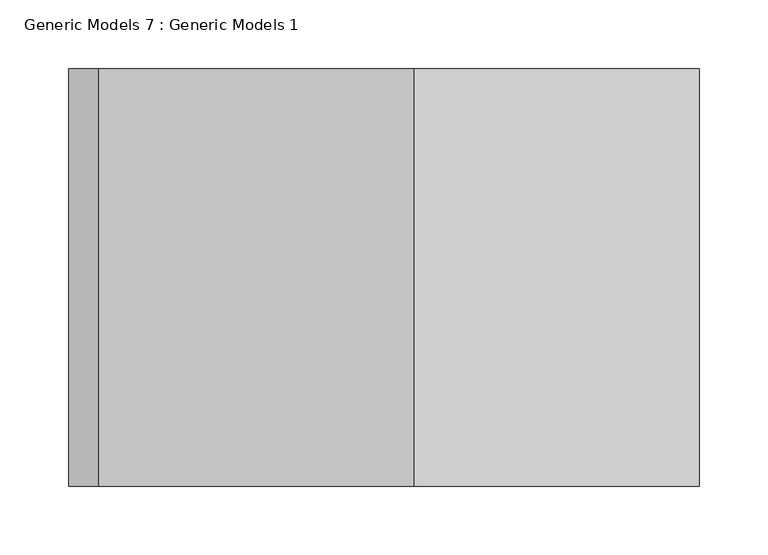
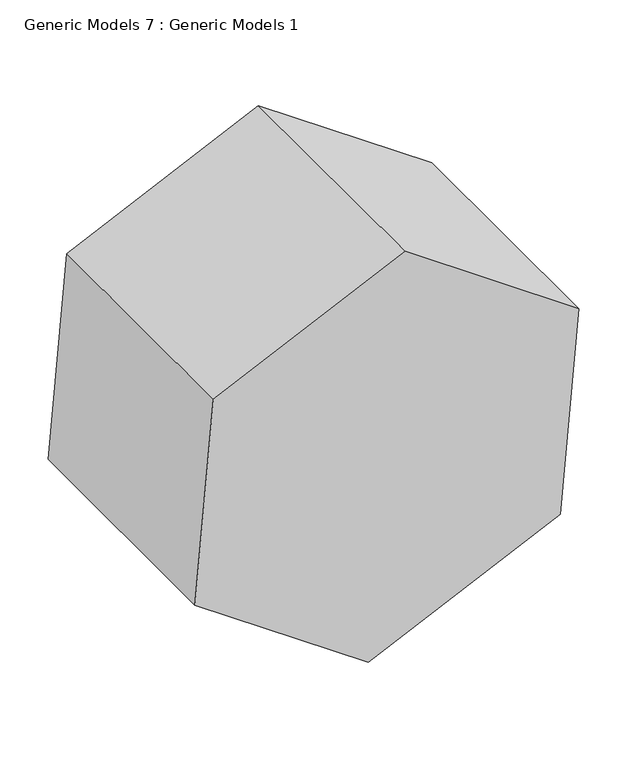
"""IFC4 building model written with IfcOpenShell, lengths in millimetres: proxy geometry, Generic Models 7 : Generic Models 1."""

from ifc_helpers import new_model, si_unit, frame, origin, place, context, project, spatial, polyline, outline, extrude, source, transform, mapped, element, save


def generic_models_7_generic_models_1_dc570d8e(model_context):
    return source(origin(), model_context, "Body", "SweptSolid", [
        extrude(outline(polyline([(833.1013393, -3000.7079055), (978.7897542, -3208.7725247), (871.4447157, -3438.9747026), (618.4112624, -3461.1122613), (472.7228475, -3253.047642), (580.067886, -3022.8454641), (833.1013393, -3000.7079055)])), frame((0.0, -10720.3372434, 0.0), z_axis=(0.0, 1.0, 0.0), x_axis=(0.0, 0.0, 1.0)), (0.0, 0.0, 1.0), 304.8),
    ])


if __name__ == "__main__":
    model = new_model("IFC4")
    model_context = context("Model", 3, world=origin())
    ifc_project = project(units=[si_unit("LENGTHUNIT", "METRE", prefix="MILLI")], contexts=[model_context])
    site = spatial("IfcSite", under=ifc_project)
    building = spatial("IfcBuilding", under=site)
    placement = place(None, origin())
    generic_models_7_generic_models_1_shape = generic_models_7_generic_models_1_dc570d8e(model_context)
    element("IfcBuildingElementProxy", 1, Name="Generic Models 7 : Generic Models 1", ObjectType="Generic Models 7 : Generic Models 1", at=placement, inside=building, context=model_context, shape_type="MappedRepresentation", body=[
        mapped(generic_models_7_generic_models_1_shape, transform((0.0, 0.0, 0.0), x_axis=(1.0, 0.0, 0.0), y_axis=(0.0, 1.0, 0.0), z_axis=(0.0, 0.0, 1.0))),
    ])
    save(model, "model.ifc")
